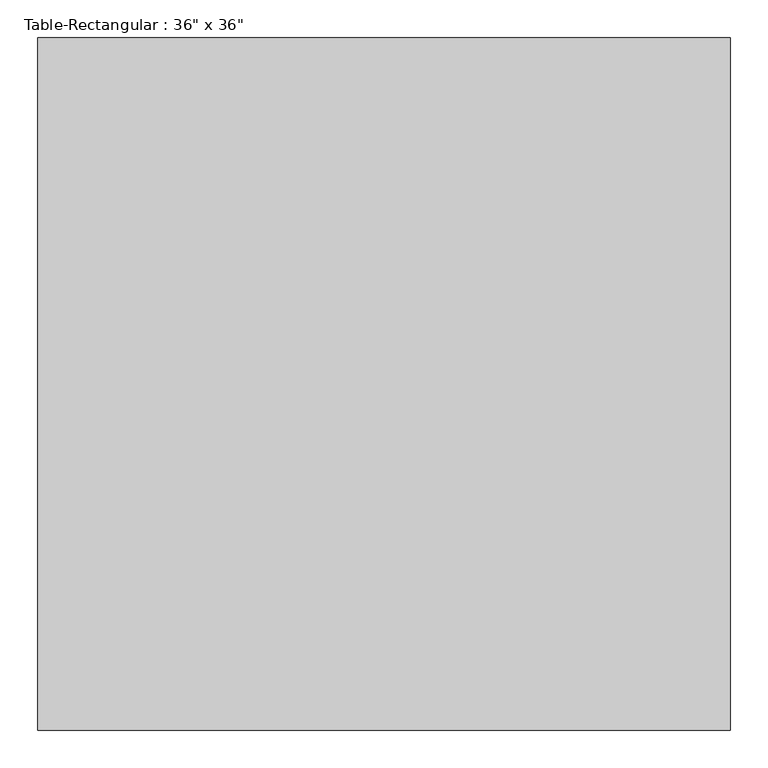
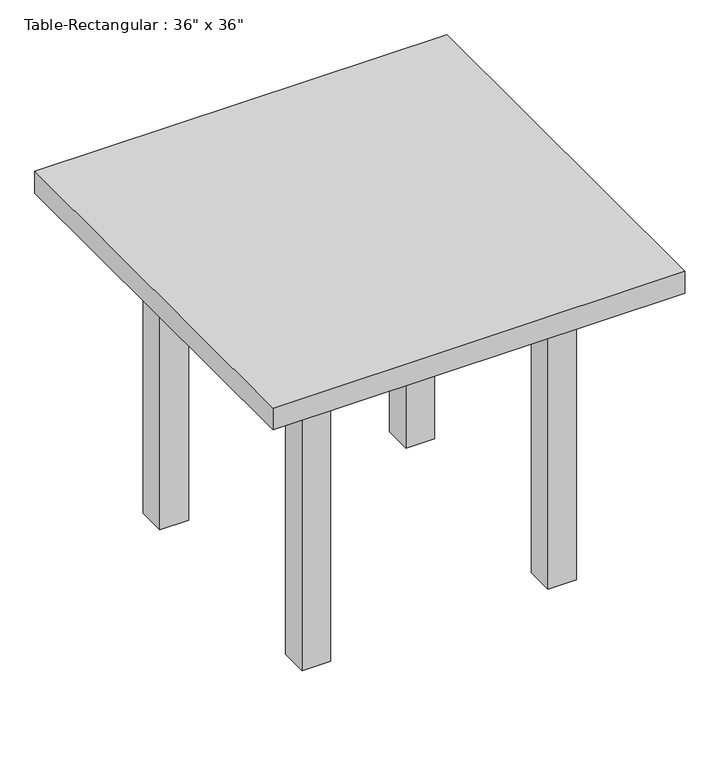
"""IFC4 building model written with IfcOpenShell, lengths in millimetres: furniture geometry."""

from ifc_helpers import new_model, si_unit, frame, origin, origin_with_axes, place, context, project, spatial, polyline, outline, extrude, source, transform, mapped, element, save


def furniture_4d44e21c(model_context):
    return source(origin(), model_context, "Body", "SweptSolid", [
        extrude(outline(polyline([(241.3, 266.7), (241.3, 241.3), (-241.3, 241.3), (-241.3, 266.7), (241.3, 266.7)])), frame((0.0, 0.0, 609.6), z_axis=(0.0, 0.0, 1.0), x_axis=(1.0, 0.0, 0.0)), (0.0, 0.0, 1.0), 101.6),
        extrude(outline(polyline([(241.3, -266.7), (-241.3, -266.7), (-241.3, -241.3), (241.3, -241.3), (241.3, -266.7)])), frame((0.0, 0.0, 609.6), z_axis=(0.0, 0.0, 1.0), x_axis=(1.0, 0.0, 0.0)), (0.0, 0.0, 1.0), 101.6),
        extrude(outline(polyline([(-254.0, -241.3), (-279.4, -241.3), (-279.4, 241.3), (-254.0, 241.3), (-254.0, -241.3)])), frame((0.0, 0.0, 609.6), z_axis=(0.0, 0.0, 1.0), x_axis=(1.0, 0.0, 0.0)), (0.0, 0.0, 1.0), 101.6),
        extrude(outline(polyline([(254.0, -241.3), (254.0, 241.3), (279.4, 241.3), (279.4, -241.3), (254.0, -241.3)])), frame((0.0, 0.0, 609.6), z_axis=(0.0, 0.0, 1.0), x_axis=(1.0, 0.0, 0.0)), (0.0, 0.0, 1.0), 101.6),
        extrude(outline(polyline([(457.2, 457.2), (457.2, -457.2), (-457.2, -457.2), (-457.2, 457.2), (457.2, 457.2)])), frame((0.0, 0.0, 711.2), z_axis=(0.0, 0.0, 1.0), x_axis=(1.0, 0.0, 0.0)), (0.0, 0.0, 1.0), 50.8),
        extrude(outline(polyline([(-241.3, 304.8), (-241.3, 241.3), (-304.8, 241.3), (-304.8, 304.8), (-241.3, 304.8)])), origin_with_axes(), (0.0, 0.0, 1.0), 711.2),
        extrude(outline(polyline([(241.3, 304.8), (304.8, 304.8), (304.8, 241.3), (241.3, 241.3), (241.3, 304.8)])), origin_with_axes(), (0.0, 0.0, 1.0), 711.2),
        extrude(outline(polyline([(-241.3, -304.8), (-304.8, -304.8), (-304.8, -241.3), (-241.3, -241.3), (-241.3, -304.8)])), origin_with_axes(), (0.0, 0.0, 1.0), 711.2),
        extrude(outline(polyline([(241.3, -304.8), (241.3, -241.3), (304.8, -241.3), (304.8, -304.8), (241.3, -304.8)])), origin_with_axes(), (0.0, 0.0, 1.0), 711.2),
    ])


if __name__ == "__main__":
    model = new_model("IFC4")
    model_context = context("Model", 3, world=origin())
    ifc_project = project(units=[si_unit("LENGTHUNIT", "METRE", prefix="MILLI")], contexts=[model_context])
    site = spatial("IfcSite", under=ifc_project)
    building = spatial("IfcBuilding", under=site)
    placement = place(None, origin())
    furniture_shape = furniture_4d44e21c(model_context)
    element("IfcFurniture", 1, ObjectType="Table-Rectangular : 36\" x 36\"", at=placement, inside=building, context=model_context, shape_type="MappedRepresentation", body=[
        mapped(furniture_shape, transform((0.0, 0.0, 0.0), x_axis=(1.0, 0.0, 0.0), y_axis=(0.0, 1.0, 0.0), z_axis=(0.0, 0.0, 1.0))),
    ])
    save(model, "model.ifc")

# Revit data of these elements
# Type "Table-Rectangular : 36\" x 36\""
#   Assembly Code = "E2020200"
#   Height = 2' - 6"
#   Length = 3' - 0"
#   Width = 3' - 0"
#   Base Material = Birch
#   Top Material = Birch
#   Default Elevation = 0
# Element 1 (IfcFurniture, "Table-Rectangular : 36\" x 36\"")
#   Materials on its faces: "Birch"
# Materials
#   "Birch": class "Wood", colour RGB 224 178 126, transparency 0, Description = "Betula Alleghaniensis", Cost = 0
